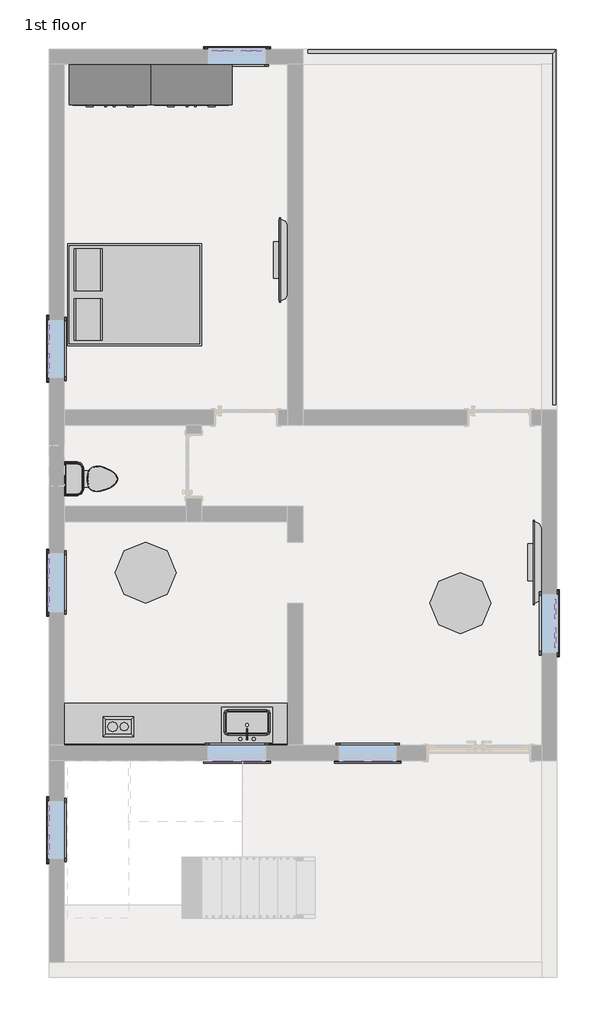
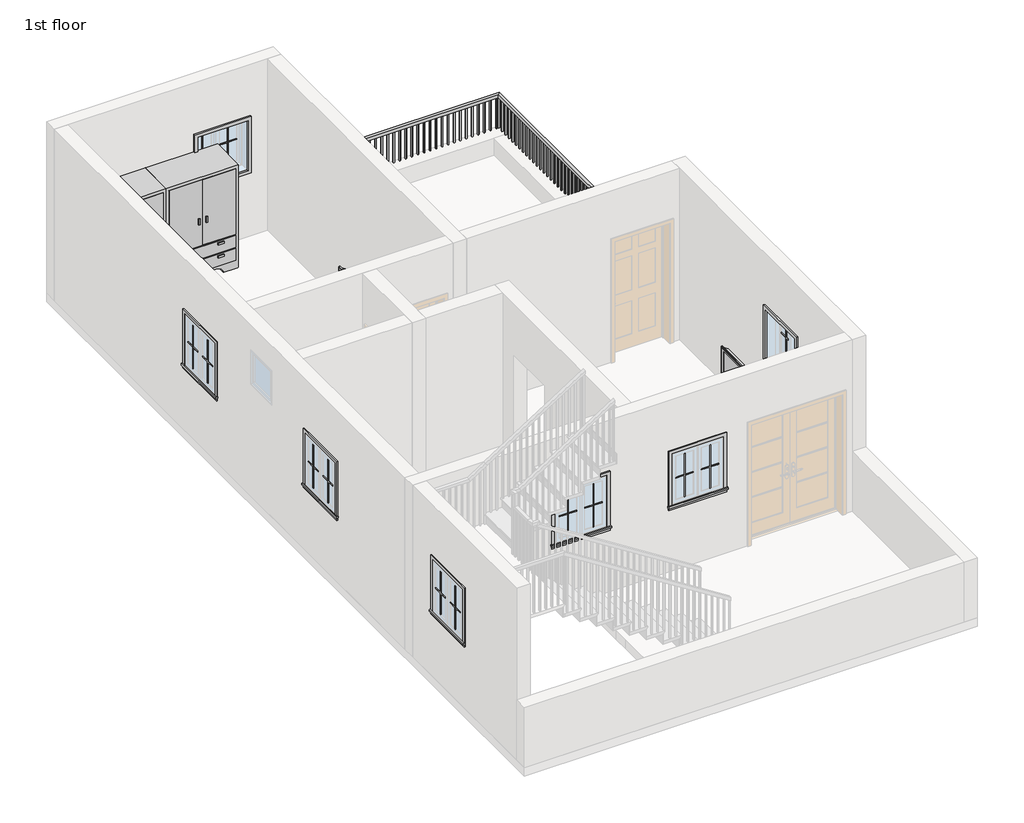
# One storey, part 3 of 3: 29 proxies, 8 furniture elements, 2 flow terminals, 1 railing.
"""IFC4 building model written with IfcOpenShell, lengths in millimetres."""

from ifc_helpers import new_model, si_unit, frame, origin, place, context, project, spatial, polyline, outline, extrude, faceted_brep, transform, mapped, element, save
from components import proxy_fb8a77b2, muntin_pattern_2x2_muntin_pattern_2x2_b3fe6957, muntin_pattern_2x2_muntin_pattern_2x2_3e0ecaf2, trim_window_exterior_flat_with_sill_41619996, trim_window_interior_flat_picture_frame_51c85655, flow_terminal_4d548711, toilet_domestic_3d_toilet_domestic_3d_ba6479b0, toilet_domestic_3d_toilet_domestic_3d_30431060, furniture_0315470b, furniture_691b2c5f, furniture_0b81fedb, furniture_ec754799, furniture_52f35bf4, furniture_82e269c4

model = new_model("IFC4")

# Units and contexts
model_context = context("Model", 3, world=origin())
ifc_project = project(units=[si_unit("LENGTHUNIT", "METRE", prefix="MILLI")], contexts=[model_context])

# Site, building, storey
site = spatial("IfcSite", under=ifc_project)
building = spatial("IfcBuilding", under=site)
storey = spatial("IfcBuildingStorey", under=building, Name="1st floor", Elevation=3810.0)

# Proxies
placement = place(None, origin())
proxy_shape = proxy_fb8a77b2(model_context)
element("IfcBuildingElementProxy", 1, Name="Cook Top-2 Unit : 12\" x 18\"", ObjectType="Cook Top-2 Unit : 12\" x 18\"", at=placement, inside=storey, context=model_context, shape_type="MappedRepresentation", body=[
    mapped(proxy_shape, transform((20084.9384757, 6960.5752787, 3810.0), x_axis=(0.0, 1.0, 0.0), y_axis=(-1.0, 0.0, 0.0), z_axis=(0.0, 0.0, 1.0))),
])
muntin_pattern_2x2_muntin_pattern_2x2_shape = muntin_pattern_2x2_muntin_pattern_2x2_b3fe6957(model_context)
element("IfcBuildingElementProxy", 2, Name="Muntin Pattern_2x2 : Muntin Pattern_2x2", ObjectType="Muntin Pattern_2x2 : Muntin Pattern_2x2", at=placement, inside=storey, context=model_context, shape_type="MappedRepresentation", body=[
    mapped(muntin_pattern_2x2_muntin_pattern_2x2_shape, transform((19022.8386801, 8981.4627787, 5064.125), x_axis=(0.0, 1.0, 0.0), y_axis=(-1.0, 0.0, 0.0), z_axis=(0.0, 0.0, 1.0))),
])
element("IfcBuildingElementProxy", 3, Name="Muntin Pattern_2x2 : Muntin Pattern_2x2", ObjectType="Muntin Pattern_2x2 : Muntin Pattern_2x2", at=placement, inside=storey, context=model_context, shape_type="MappedRepresentation", body=[
    mapped(muntin_pattern_2x2_muntin_pattern_2x2_shape, transform((19022.8386801, 12486.6627787, 5064.125), x_axis=(0.0, 1.0, 0.0), y_axis=(-1.0, 0.0, 0.0), z_axis=(0.0, 0.0, 1.0))),
])
element("IfcBuildingElementProxy", 4, Name="Muntin Pattern_2x2 : Muntin Pattern_2x2", ObjectType="Muntin Pattern_2x2 : Muntin Pattern_2x2", at=placement, inside=storey, context=model_context, shape_type="MappedRepresentation", body=[
    mapped(muntin_pattern_2x2_muntin_pattern_2x2_shape, transform((26623.7886801, 8800.4877787, 5064.125), x_axis=(0.0, -1.0, 0.0), y_axis=(1.0, 0.0, 0.0), z_axis=(0.0, 0.0, 1.0))),
])
element("IfcBuildingElementProxy", 5, Name="Muntin Pattern_2x2 : Muntin Pattern_2x2", ObjectType="Muntin Pattern_2x2 : Muntin Pattern_2x2", at=placement, inside=storey, context=model_context, shape_type="MappedRepresentation", body=[
    mapped(muntin_pattern_2x2_muntin_pattern_2x2_shape, transform((21618.4011801, 17187.2502787, 5064.125), x_axis=(1.0, 0.0, 0.0), y_axis=(0.0, 1.0, 0.0), z_axis=(0.0, 0.0, 1.0))),
])
element("IfcBuildingElementProxy", 6, Name="Muntin Pattern_2x2 : Muntin Pattern_2x2", ObjectType="Muntin Pattern_2x2 : Muntin Pattern_2x2", at=placement, inside=storey, context=model_context, shape_type="MappedRepresentation", body=[
    mapped(muntin_pattern_2x2_muntin_pattern_2x2_shape, transform((22047.0261801, 6538.3002787, 5064.125), x_axis=(-1.0, 0.0, 0.0), y_axis=(0.0, -1.0, 0.0), z_axis=(0.0, 0.0, 1.0))),
])
element("IfcBuildingElementProxy", 7, Name="Muntin Pattern_2x2 : Muntin Pattern_2x2", ObjectType="Muntin Pattern_2x2 : Muntin Pattern_2x2", at=placement, inside=storey, context=model_context, shape_type="MappedRepresentation", body=[
    mapped(muntin_pattern_2x2_muntin_pattern_2x2_shape, transform((24009.1761801, 6538.3002787, 5064.125), x_axis=(-1.0, 0.0, 0.0), y_axis=(0.0, -1.0, 0.0), z_axis=(0.0, 0.0, 1.0))),
])
element("IfcBuildingElementProxy", 8, Name="Muntin Pattern_2x2 : Muntin Pattern_2x2", ObjectType="Muntin Pattern_2x2 : Muntin Pattern_2x2", at=placement, inside=storey, context=model_context, shape_type="MappedRepresentation", body=[
    mapped(muntin_pattern_2x2_muntin_pattern_2x2_shape, transform((19022.8386801, 5273.0627787, 5064.125), x_axis=(0.0, 1.0, 0.0), y_axis=(-1.0, 0.0, 0.0), z_axis=(0.0, 0.0, 1.0))),
])
muntin_pattern_2x2_muntin_pattern_2x2_2_shape = muntin_pattern_2x2_muntin_pattern_2x2_3e0ecaf2(model_context)
element("IfcBuildingElementProxy", 9, Name="Muntin Pattern_2x2 : Muntin Pattern_2x2", ObjectType="Muntin Pattern_2x2 : Muntin Pattern_2x2", at=placement, inside=storey, context=model_context, shape_type="MappedRepresentation", body=[
    mapped(muntin_pattern_2x2_muntin_pattern_2x2_2_shape, transform((19022.8386801, 9410.0877787, 5064.125), x_axis=(0.0, -1.0, 0.0), y_axis=(1.0, 0.0, 0.0), z_axis=(0.0, 0.0, 1.0))),
])
element("IfcBuildingElementProxy", 10, Name="Muntin Pattern_2x2 : Muntin Pattern_2x2", ObjectType="Muntin Pattern_2x2 : Muntin Pattern_2x2", at=placement, inside=storey, context=model_context, shape_type="MappedRepresentation", body=[
    mapped(muntin_pattern_2x2_muntin_pattern_2x2_2_shape, transform((19022.8386801, 12915.2877787, 5064.125), x_axis=(0.0, -1.0, 0.0), y_axis=(1.0, 0.0, 0.0), z_axis=(0.0, 0.0, 1.0))),
])
element("IfcBuildingElementProxy", 11, Name="Muntin Pattern_2x2 : Muntin Pattern_2x2", ObjectType="Muntin Pattern_2x2 : Muntin Pattern_2x2", at=placement, inside=storey, context=model_context, shape_type="MappedRepresentation", body=[
    mapped(muntin_pattern_2x2_muntin_pattern_2x2_2_shape, transform((26623.7886801, 8371.8627787, 5064.125), x_axis=(0.0, 1.0, 0.0), y_axis=(-1.0, 0.0, 0.0), z_axis=(0.0, 0.0, 1.0))),
])
element("IfcBuildingElementProxy", 12, Name="Muntin Pattern_2x2 : Muntin Pattern_2x2", ObjectType="Muntin Pattern_2x2 : Muntin Pattern_2x2", at=placement, inside=storey, context=model_context, shape_type="MappedRepresentation", body=[
    mapped(muntin_pattern_2x2_muntin_pattern_2x2_2_shape, transform((22047.0261801, 17187.2502787, 5064.125), x_axis=(-1.0, 0.0, 0.0), y_axis=(0.0, -1.0, 0.0), z_axis=(0.0, 0.0, 1.0))),
])
element("IfcBuildingElementProxy", 13, Name="Muntin Pattern_2x2 : Muntin Pattern_2x2", ObjectType="Muntin Pattern_2x2 : Muntin Pattern_2x2", at=placement, inside=storey, context=model_context, shape_type="MappedRepresentation", body=[
    mapped(muntin_pattern_2x2_muntin_pattern_2x2_2_shape, transform((21618.4011801, 6538.3002787, 5064.125), x_axis=(1.0, 0.0, 0.0), y_axis=(0.0, 1.0, 0.0), z_axis=(0.0, 0.0, 1.0))),
])
element("IfcBuildingElementProxy", 14, Name="Muntin Pattern_2x2 : Muntin Pattern_2x2", ObjectType="Muntin Pattern_2x2 : Muntin Pattern_2x2", at=placement, inside=storey, context=model_context, shape_type="MappedRepresentation", body=[
    mapped(muntin_pattern_2x2_muntin_pattern_2x2_2_shape, transform((23580.5511801, 6538.3002787, 5064.125), x_axis=(1.0, 0.0, 0.0), y_axis=(0.0, 1.0, 0.0), z_axis=(0.0, 0.0, 1.0))),
])
element("IfcBuildingElementProxy", 15, Name="Muntin Pattern_2x2 : Muntin Pattern_2x2", ObjectType="Muntin Pattern_2x2 : Muntin Pattern_2x2", at=placement, inside=storey, context=model_context, shape_type="MappedRepresentation", body=[
    mapped(muntin_pattern_2x2_muntin_pattern_2x2_2_shape, transform((19022.8386801, 5701.6877787, 5064.125), x_axis=(0.0, -1.0, 0.0), y_axis=(1.0, 0.0, 0.0), z_axis=(0.0, 0.0, 1.0))),
])
trim_window_exterior_flat_with_sill_shape = trim_window_exterior_flat_with_sill_41619996(model_context)
element("IfcBuildingElementProxy", 16, Name="Trim-Window-Exterior-Flat : with Sill", ObjectType="Trim-Window-Exterior-Flat : with Sill", at=placement, inside=storey, context=model_context, shape_type="MappedRepresentation", body=[
    mapped(trim_window_exterior_flat_with_sill_shape, transform((19013.3136801, 9195.7752787, 5908.675), x_axis=(0.0, -1.0, 0.0), y_axis=(0.0, 0.0, 1.0), z_axis=(-1.0, 0.0, 0.0))),
])
element("IfcBuildingElementProxy", 17, Name="Trim-Window-Exterior-Flat : with Sill", ObjectType="Trim-Window-Exterior-Flat : with Sill", at=placement, inside=storey, context=model_context, shape_type="MappedRepresentation", body=[
    mapped(trim_window_exterior_flat_with_sill_shape, transform((19013.3136801, 12700.9752787, 5908.675), x_axis=(0.0, -1.0, 0.0), y_axis=(0.0, 0.0, 1.0), z_axis=(-1.0, 0.0, 0.0))),
])
element("IfcBuildingElementProxy", 18, Name="Trim-Window-Exterior-Flat : with Sill", ObjectType="Trim-Window-Exterior-Flat : with Sill", at=placement, inside=storey, context=model_context, shape_type="MappedRepresentation", body=[
    mapped(trim_window_exterior_flat_with_sill_shape, transform((26633.3136801, 8586.1752787, 5908.675), x_axis=(0.0, 1.0, 0.0), y_axis=(0.0, 0.0, 1.0), z_axis=(1.0, 0.0, 0.0))),
])
element("IfcBuildingElementProxy", 19, Name="Trim-Window-Exterior-Flat : with Sill", ObjectType="Trim-Window-Exterior-Flat : with Sill", at=placement, inside=storey, context=model_context, shape_type="MappedRepresentation", body=[
    mapped(trim_window_exterior_flat_with_sill_shape, transform((21832.7136801, 17196.7752787, 5908.675), x_axis=(-1.0, 0.0, 0.0), y_axis=(0.0, 0.0, 1.0), z_axis=(0.0, 1.0, 0.0))),
])
element("IfcBuildingElementProxy", 20, Name="Trim-Window-Exterior-Flat : with Sill", ObjectType="Trim-Window-Exterior-Flat : with Sill", at=placement, inside=storey, context=model_context, shape_type="MappedRepresentation", body=[
    mapped(trim_window_exterior_flat_with_sill_shape, transform((21832.7136801, 6528.7752787, 5908.675), x_axis=(1.0, 0.0, 0.0), y_axis=(0.0, 0.0, 1.0), z_axis=(0.0, -1.0, 0.0))),
])
element("IfcBuildingElementProxy", 21, Name="Trim-Window-Exterior-Flat : with Sill", ObjectType="Trim-Window-Exterior-Flat : with Sill", at=placement, inside=storey, context=model_context, shape_type="MappedRepresentation", body=[
    mapped(trim_window_exterior_flat_with_sill_shape, transform((23794.8636801, 6528.7752787, 5908.675), x_axis=(1.0, 0.0, 0.0), y_axis=(0.0, 0.0, 1.0), z_axis=(0.0, -1.0, 0.0))),
])
element("IfcBuildingElementProxy", 22, Name="Trim-Window-Exterior-Flat : with Sill", ObjectType="Trim-Window-Exterior-Flat : with Sill", at=placement, inside=storey, context=model_context, shape_type="MappedRepresentation", body=[
    mapped(trim_window_exterior_flat_with_sill_shape, transform((19013.3136801, 5487.3752787, 5908.675), x_axis=(0.0, -1.0, 0.0), y_axis=(0.0, 0.0, 1.0), z_axis=(-1.0, 0.0, 0.0))),
])
trim_window_interior_flat_picture_frame_shape = trim_window_interior_flat_picture_frame_51c85655(model_context)
element("IfcBuildingElementProxy", 23, Name="Trim-Window-Interior-Flat : Picture Frame", ObjectType="Trim-Window-Interior-Flat : Picture Frame", at=placement, inside=storey, context=model_context, shape_type="MappedRepresentation", body=[
    mapped(trim_window_interior_flat_picture_frame_shape, transform((19241.9136801, 9195.7752787, 5908.675), x_axis=(0.0, 1.0, 0.0), y_axis=(0.0, 0.0, 1.0), z_axis=(1.0, 0.0, 0.0))),
])
element("IfcBuildingElementProxy", 24, Name="Trim-Window-Interior-Flat : Picture Frame", ObjectType="Trim-Window-Interior-Flat : Picture Frame", at=placement, inside=storey, context=model_context, shape_type="MappedRepresentation", body=[
    mapped(trim_window_interior_flat_picture_frame_shape, transform((19241.9136801, 12700.9752787, 5908.675), x_axis=(0.0, 1.0, 0.0), y_axis=(0.0, 0.0, 1.0), z_axis=(1.0, 0.0, 0.0))),
])
element("IfcBuildingElementProxy", 25, Name="Trim-Window-Interior-Flat : Picture Frame", ObjectType="Trim-Window-Interior-Flat : Picture Frame", at=placement, inside=storey, context=model_context, shape_type="MappedRepresentation", body=[
    mapped(trim_window_interior_flat_picture_frame_shape, transform((26404.7136801, 8586.1752787, 5908.675), x_axis=(0.0, -1.0, 0.0), y_axis=(0.0, 0.0, 1.0), z_axis=(-1.0, 0.0, 0.0))),
])
element("IfcBuildingElementProxy", 26, Name="Trim-Window-Interior-Flat : Picture Frame", ObjectType="Trim-Window-Interior-Flat : Picture Frame", at=placement, inside=storey, context=model_context, shape_type="MappedRepresentation", body=[
    mapped(trim_window_interior_flat_picture_frame_shape, transform((21832.7136801, 16968.1752787, 5908.675), x_axis=(1.0, 0.0, 0.0), y_axis=(0.0, 0.0, 1.0), z_axis=(0.0, -1.0, 0.0))),
])
element("IfcBuildingElementProxy", 27, Name="Trim-Window-Interior-Flat : Picture Frame", ObjectType="Trim-Window-Interior-Flat : Picture Frame", at=placement, inside=storey, context=model_context, shape_type="MappedRepresentation", body=[
    mapped(trim_window_interior_flat_picture_frame_shape, transform((21832.7136801, 6757.3752787, 5908.675), x_axis=(-1.0, 0.0, 0.0), y_axis=(0.0, 0.0, 1.0), z_axis=(0.0, 1.0, 0.0))),
])
element("IfcBuildingElementProxy", 28, Name="Trim-Window-Interior-Flat : Picture Frame", ObjectType="Trim-Window-Interior-Flat : Picture Frame", at=placement, inside=storey, context=model_context, shape_type="MappedRepresentation", body=[
    mapped(trim_window_interior_flat_picture_frame_shape, transform((23794.8636801, 6757.3752787, 5908.675), x_axis=(-1.0, 0.0, 0.0), y_axis=(0.0, 0.0, 1.0), z_axis=(0.0, 1.0, 0.0))),
])
element("IfcBuildingElementProxy", 29, Name="Trim-Window-Interior-Flat : Picture Frame", ObjectType="Trim-Window-Interior-Flat : Picture Frame", at=placement, inside=storey, context=model_context, shape_type="MappedRepresentation", body=[
    mapped(trim_window_interior_flat_picture_frame_shape, transform((19241.9136801, 5487.3752787, 5908.675), x_axis=(0.0, 1.0, 0.0), y_axis=(0.0, 0.0, 1.0), z_axis=(1.0, 0.0, 0.0))),
])

# Flow terminals
flow_terminal_shape = flow_terminal_4d548711(model_context)
element("IfcFlowTerminal", 30, ObjectType="Sink Kitchen-Single : 30\" x 21\"", at=placement, inside=storey, context=model_context, shape_type="MappedRepresentation", body=[
    mapped(flow_terminal_shape, transform((22000.8029206, 7064.5206798, 3810.0), x_axis=(-1.0, 0.0, 0.0), y_axis=(0.0, -1.0, 0.0), z_axis=(0.0, 0.0, 1.0))),
])
toilet_domestic_3d_toilet_domestic_3d_shape = toilet_domestic_3d_toilet_domestic_3d_ba6479b0(model_context)
toilet_domestic_3d_toilet_domestic_3d_2_shape = toilet_domestic_3d_toilet_domestic_3d_30431060(model_context)
element("IfcFlowTerminal", 31, ObjectType="Toilet-Domestic-3D : Toilet-Domestic-3D", at=placement, inside=storey, context=model_context, shape_type="MappedRepresentation", body=[
    mapped(toilet_domestic_3d_toilet_domestic_3d_shape, transform((19736.6097074, 10752.6409313, 3810.0), x_axis=(0.0, 1.0, 0.0), y_axis=(-1.0, 0.0, 0.0), z_axis=(0.0, 0.0, 1.0))),
    mapped(toilet_domestic_3d_toilet_domestic_3d_2_shape, transform((19736.6097074, 10752.6409313, 3810.0), x_axis=(0.0, 1.0, 0.0), y_axis=(-1.0, 0.0, 0.0), z_axis=(0.0, 0.0, 1.0))),
])

# Furniture
furniture_shape = furniture_0315470b(model_context)
element("IfcFurniture", 32, ObjectType="Bed-Box : Queen 60\" x 79\"", at=placement, inside=storey, context=model_context, shape_type="MappedRepresentation", body=[
    mapped(furniture_shape, transform((20061.5841719, 13174.6228197, 3810.0), x_axis=(0.0, 1.0, 0.0), y_axis=(-1.0, 0.0, 0.0), z_axis=(0.0, 0.0, 1.0))),
])
furniture_2_shape = furniture_691b2c5f(model_context)
element("IfcFurniture", 33, ObjectType="Counter Top w Sink Hole : 24\" Depth", at=placement, inside=storey, context=model_context, shape_type="MappedRepresentation", body=[
    mapped(furniture_2_shape, transform((21394.251385, 6757.3752787, 3810.0), x_axis=(-1.0, 0.0, 0.0), y_axis=(0.0, -1.0, 0.0), z_axis=(0.0, 0.0, 1.0))),
])
furniture_3_shape = furniture_0b81fedb(model_context)
element("IfcFurniture", 34, ObjectType="TV - Flat Screen : 50\"", at=placement, inside=storey, context=model_context, shape_type="MappedRepresentation", body=[
    mapped(furniture_3_shape, transform((26346.1750564, 9496.6307646, 3810.0), x_axis=(0.0, -1.0, 0.0), y_axis=(1.0, 0.0, 0.0), z_axis=(0.0, 0.0, 1.0))),
])
element("IfcFurniture", 35, ObjectType="TV - Flat Screen : 50\"", at=placement, inside=storey, context=model_context, shape_type="MappedRepresentation", body=[
    mapped(furniture_3_shape, transform((22536.1750564, 14030.5307646, 3810.0), x_axis=(0.0, -1.0, 0.0), y_axis=(1.0, 0.0, 0.0), z_axis=(0.0, 0.0, 1.0))),
])
furniture_4_shape = furniture_ec754799(model_context)
element("IfcFurniture", 36, ObjectType="Table-Dining Round : 36\" Diameter", at=placement, inside=storey, context=model_context, shape_type="MappedRepresentation", body=[
    mapped(furniture_4_shape, transform((25081.8317129, 9075.8539672, 3810.0), x_axis=(1.0, 0.0, 0.0), y_axis=(0.0, 1.0, 0.0), z_axis=(0.0, 0.0, 1.0))),
])
furniture_5_shape = furniture_52f35bf4(model_context)
element("IfcFurniture", 37, ObjectType="Table-Dining Round w Chairs : 36\" Diameter", at=placement, inside=storey, context=model_context, shape_type="MappedRepresentation", body=[
    mapped(furniture_5_shape, transform((20357.4317129, 9533.0539672, 3810.0), x_axis=(1.0, 0.0, 0.0), y_axis=(0.0, 1.0, 0.0), z_axis=(0.0, 0.0, 1.0))),
])
furniture_6_shape = furniture_82e269c4(model_context)
element("IfcFurniture", 38, ObjectType="Wardrobe : 48\" x 72\" x 24\"", at=placement, inside=storey, context=model_context, shape_type="MappedRepresentation", body=[
    mapped(furniture_6_shape, transform((20196.9069399, 17247.1140883, 3810.0), x_axis=(1.0, 0.0, 0.0), y_axis=(0.0, 1.0, 0.0), z_axis=(0.0, 0.0, 1.0))),
])
element("IfcFurniture", 39, ObjectType="Wardrobe : 48\" x 72\" x 24\"", at=placement, inside=storey, context=model_context, shape_type="MappedRepresentation", body=[
    mapped(furniture_6_shape, transform((21416.1069399, 17247.1140883, 3810.0), x_axis=(1.0, 0.0, 0.0), y_axis=(0.0, 1.0, 0.0), z_axis=(0.0, 0.0, 1.0))),
])

# Railing
element("IfcRailing", 40, ObjectType="Handrail - Rectangular", at=placement, inside=storey, context=model_context, shape_type="SolidModel", body=[
    faceted_brep([(22899.5136801, 17184.0752787, 4724.4), (22899.5136801, 17184.0752787, 4673.6), (22899.5136801, 17133.2752787, 4673.6), (22899.5136801, 17133.2752787, 4724.4), (26620.6136801, 17184.0752787, 4724.4), (26620.6136801, 17184.0752787, 4673.6), (26569.8136801, 17133.2752787, 4673.6), (26569.8136801, 17133.2752787, 4724.4), (26620.6136801, 11862.7752787, 4724.4), (26569.8136801, 11862.7752787, 4724.4), (26569.8136801, 11862.7752787, 4673.6), (26620.6136801, 11862.7752787, 4673.6)], [[[0, 1, 2, 3]], [[1, 0, 4, 5]], [[2, 1, 5, 6]], [[3, 2, 6, 7]], [[0, 3, 7, 4]], [[8, 9, 10, 11]], [[5, 4, 8, 11]], [[6, 5, 11, 10]], [[7, 6, 10, 9]], [[4, 7, 9, 8]]]),
    extrude(outline(polyline([(26604.7386801, 11885.0002787), (26604.7386801, 11865.9502787), (26585.6886801, 11865.9502787), (26585.6886801, 11885.0002787), (26604.7386801, 11885.0002787)])), frame((0.0, 0.0, 3810.0), z_axis=(0.0, 0.0, 1.0), x_axis=(1.0, 0.0, 0.0)), (0.0, 0.0, 1.0), 863.6),
    extrude(outline(polyline([(26604.7386801, 11986.6002787), (26604.7386801, 11967.5502787), (26585.6886801, 11967.5502787), (26585.6886801, 11986.6002787), (26604.7386801, 11986.6002787)])), frame((0.0, 0.0, 3810.0), z_axis=(0.0, 0.0, 1.0), x_axis=(1.0, 0.0, 0.0)), (0.0, 0.0, 1.0), 863.6),
    extrude(outline(polyline([(26604.7386801, 12088.2002787), (26604.7386801, 12069.1502787), (26585.6886801, 12069.1502787), (26585.6886801, 12088.2002787), (26604.7386801, 12088.2002787)])), frame((0.0, 0.0, 3810.0), z_axis=(0.0, 0.0, 1.0), x_axis=(1.0, 0.0, 0.0)), (0.0, 0.0, 1.0), 863.6),
    extrude(outline(polyline([(26604.7386801, 12189.8002787), (26604.7386801, 12170.7502787), (26585.6886801, 12170.7502787), (26585.6886801, 12189.8002787), (26604.7386801, 12189.8002787)])), frame((0.0, 0.0, 3810.0), z_axis=(0.0, 0.0, 1.0), x_axis=(1.0, 0.0, 0.0)), (0.0, 0.0, 1.0), 863.6),
    extrude(outline(polyline([(26604.7386801, 12291.4002787), (26604.7386801, 12272.3502787), (26585.6886801, 12272.3502787), (26585.6886801, 12291.4002787), (26604.7386801, 12291.4002787)])), frame((0.0, 0.0, 3810.0), z_axis=(0.0, 0.0, 1.0), x_axis=(1.0, 0.0, 0.0)), (0.0, 0.0, 1.0), 863.6),
    extrude(outline(polyline([(26604.7386801, 12393.0002787), (26604.7386801, 12373.9502787), (26585.6886801, 12373.9502787), (26585.6886801, 12393.0002787), (26604.7386801, 12393.0002787)])), frame((0.0, 0.0, 3810.0), z_axis=(0.0, 0.0, 1.0), x_axis=(1.0, 0.0, 0.0)), (0.0, 0.0, 1.0), 863.6),
    extrude(outline(polyline([(26604.7386801, 12494.6002787), (26604.7386801, 12475.5502787), (26585.6886801, 12475.5502787), (26585.6886801, 12494.6002787), (26604.7386801, 12494.6002787)])), frame((0.0, 0.0, 3810.0), z_axis=(0.0, 0.0, 1.0), x_axis=(1.0, 0.0, 0.0)), (0.0, 0.0, 1.0), 863.6),
    extrude(outline(polyline([(26604.7386801, 12596.2002787), (26604.7386801, 12577.1502787), (26585.6886801, 12577.1502787), (26585.6886801, 12596.2002787), (26604.7386801, 12596.2002787)])), frame((0.0, 0.0, 3810.0), z_axis=(0.0, 0.0, 1.0), x_axis=(1.0, 0.0, 0.0)), (0.0, 0.0, 1.0), 863.6),
    extrude(outline(polyline([(26604.7386801, 12697.8002787), (26604.7386801, 12678.7502787), (26585.6886801, 12678.7502787), (26585.6886801, 12697.8002787), (26604.7386801, 12697.8002787)])), frame((0.0, 0.0, 3810.0), z_axis=(0.0, 0.0, 1.0), x_axis=(1.0, 0.0, 0.0)), (0.0, 0.0, 1.0), 863.6),
    extrude(outline(polyline([(26604.7386801, 12799.4002787), (26604.7386801, 12780.3502787), (26585.6886801, 12780.3502787), (26585.6886801, 12799.4002787), (26604.7386801, 12799.4002787)])), frame((0.0, 0.0, 3810.0), z_axis=(0.0, 0.0, 1.0), x_axis=(1.0, 0.0, 0.0)), (0.0, 0.0, 1.0), 863.6),
    extrude(outline(polyline([(26604.7386801, 12901.0002787), (26604.7386801, 12881.9502787), (26585.6886801, 12881.9502787), (26585.6886801, 12901.0002787), (26604.7386801, 12901.0002787)])), frame((0.0, 0.0, 3810.0), z_axis=(0.0, 0.0, 1.0), x_axis=(1.0, 0.0, 0.0)), (0.0, 0.0, 1.0), 863.6),
    extrude(outline(polyline([(26604.7386801, 13002.6002787), (26604.7386801, 12983.5502787), (26585.6886801, 12983.5502787), (26585.6886801, 13002.6002787), (26604.7386801, 13002.6002787)])), frame((0.0, 0.0, 3810.0), z_axis=(0.0, 0.0, 1.0), x_axis=(1.0, 0.0, 0.0)), (0.0, 0.0, 1.0), 863.6),
    extrude(outline(polyline([(26604.7386801, 13104.2002787), (26604.7386801, 13085.1502787), (26585.6886801, 13085.1502787), (26585.6886801, 13104.2002787), (26604.7386801, 13104.2002787)])), frame((0.0, 0.0, 3810.0), z_axis=(0.0, 0.0, 1.0), x_axis=(1.0, 0.0, 0.0)), (0.0, 0.0, 1.0), 863.6),
    extrude(outline(polyline([(26604.7386801, 13205.8002787), (26604.7386801, 13186.7502787), (26585.6886801, 13186.7502787), (26585.6886801, 13205.8002787), (26604.7386801, 13205.8002787)])), frame((0.0, 0.0, 3810.0), z_axis=(0.0, 0.0, 1.0), x_axis=(1.0, 0.0, 0.0)), (0.0, 0.0, 1.0), 863.6),
    extrude(outline(polyline([(26604.7386801, 13307.4002787), (26604.7386801, 13288.3502787), (26585.6886801, 13288.3502787), (26585.6886801, 13307.4002787), (26604.7386801, 13307.4002787)])), frame((0.0, 0.0, 3810.0), z_axis=(0.0, 0.0, 1.0), x_axis=(1.0, 0.0, 0.0)), (0.0, 0.0, 1.0), 863.6),
    extrude(outline(polyline([(26604.7386801, 13409.0002787), (26604.7386801, 13389.9502787), (26585.6886801, 13389.9502787), (26585.6886801, 13409.0002787), (26604.7386801, 13409.0002787)])), frame((0.0, 0.0, 3810.0), z_axis=(0.0, 0.0, 1.0), x_axis=(1.0, 0.0, 0.0)), (0.0, 0.0, 1.0), 863.6),
    extrude(outline(polyline([(26604.7386801, 13510.6002787), (26604.7386801, 13491.5502787), (26585.6886801, 13491.5502787), (26585.6886801, 13510.6002787), (26604.7386801, 13510.6002787)])), frame((0.0, 0.0, 3810.0), z_axis=(0.0, 0.0, 1.0), x_axis=(1.0, 0.0, 0.0)), (0.0, 0.0, 1.0), 863.6),
    extrude(outline(polyline([(26604.7386801, 13612.2002787), (26604.7386801, 13593.1502787), (26585.6886801, 13593.1502787), (26585.6886801, 13612.2002787), (26604.7386801, 13612.2002787)])), frame((0.0, 0.0, 3810.0), z_axis=(0.0, 0.0, 1.0), x_axis=(1.0, 0.0, 0.0)), (0.0, 0.0, 1.0), 863.6),
    extrude(outline(polyline([(26604.7386801, 13713.8002787), (26604.7386801, 13694.7502787), (26585.6886801, 13694.7502787), (26585.6886801, 13713.8002787), (26604.7386801, 13713.8002787)])), frame((0.0, 0.0, 3810.0), z_axis=(0.0, 0.0, 1.0), x_axis=(1.0, 0.0, 0.0)), (0.0, 0.0, 1.0), 863.6),
    extrude(outline(polyline([(26604.7386801, 13815.4002787), (26604.7386801, 13796.3502787), (26585.6886801, 13796.3502787), (26585.6886801, 13815.4002787), (26604.7386801, 13815.4002787)])), frame((0.0, 0.0, 3810.0), z_axis=(0.0, 0.0, 1.0), x_axis=(1.0, 0.0, 0.0)), (0.0, 0.0, 1.0), 863.6),
    extrude(outline(polyline([(26604.7386801, 13917.0002787), (26604.7386801, 13897.9502787), (26585.6886801, 13897.9502787), (26585.6886801, 13917.0002787), (26604.7386801, 13917.0002787)])), frame((0.0, 0.0, 3810.0), z_axis=(0.0, 0.0, 1.0), x_axis=(1.0, 0.0, 0.0)), (0.0, 0.0, 1.0), 863.6),
    extrude(outline(polyline([(26604.7386801, 14018.6002787), (26604.7386801, 13999.5502787), (26585.6886801, 13999.5502787), (26585.6886801, 14018.6002787), (26604.7386801, 14018.6002787)])), frame((0.0, 0.0, 3810.0), z_axis=(0.0, 0.0, 1.0), x_axis=(1.0, 0.0, 0.0)), (0.0, 0.0, 1.0), 863.6),
    extrude(outline(polyline([(26604.7386801, 14120.2002787), (26604.7386801, 14101.1502787), (26585.6886801, 14101.1502787), (26585.6886801, 14120.2002787), (26604.7386801, 14120.2002787)])), frame((0.0, 0.0, 3810.0), z_axis=(0.0, 0.0, 1.0), x_axis=(1.0, 0.0, 0.0)), (0.0, 0.0, 1.0), 863.6),
    extrude(outline(polyline([(26604.7386801, 14221.8002787), (26604.7386801, 14202.7502787), (26585.6886801, 14202.7502787), (26585.6886801, 14221.8002787), (26604.7386801, 14221.8002787)])), frame((0.0, 0.0, 3810.0), z_axis=(0.0, 0.0, 1.0), x_axis=(1.0, 0.0, 0.0)), (0.0, 0.0, 1.0), 863.6),
    extrude(outline(polyline([(26604.7386801, 14323.4002787), (26604.7386801, 14304.3502787), (26585.6886801, 14304.3502787), (26585.6886801, 14323.4002787), (26604.7386801, 14323.4002787)])), frame((0.0, 0.0, 3810.0), z_axis=(0.0, 0.0, 1.0), x_axis=(1.0, 0.0, 0.0)), (0.0, 0.0, 1.0), 863.6),
    extrude(outline(polyline([(26604.7386801, 14425.0002787), (26604.7386801, 14405.9502787), (26585.6886801, 14405.9502787), (26585.6886801, 14425.0002787), (26604.7386801, 14425.0002787)])), frame((0.0, 0.0, 3810.0), z_axis=(0.0, 0.0, 1.0), x_axis=(1.0, 0.0, 0.0)), (0.0, 0.0, 1.0), 863.6),
    extrude(outline(polyline([(26604.7386801, 14526.6002787), (26604.7386801, 14507.5502787), (26585.6886801, 14507.5502787), (26585.6886801, 14526.6002787), (26604.7386801, 14526.6002787)])), frame((0.0, 0.0, 3810.0), z_axis=(0.0, 0.0, 1.0), x_axis=(1.0, 0.0, 0.0)), (0.0, 0.0, 1.0), 863.6),
    extrude(outline(polyline([(26604.7386801, 14628.2002787), (26604.7386801, 14609.1502787), (26585.6886801, 14609.1502787), (26585.6886801, 14628.2002787), (26604.7386801, 14628.2002787)])), frame((0.0, 0.0, 3810.0), z_axis=(0.0, 0.0, 1.0), x_axis=(1.0, 0.0, 0.0)), (0.0, 0.0, 1.0), 863.6),
    extrude(outline(polyline([(26604.7386801, 14729.8002787), (26604.7386801, 14710.7502787), (26585.6886801, 14710.7502787), (26585.6886801, 14729.8002787), (26604.7386801, 14729.8002787)])), frame((0.0, 0.0, 3810.0), z_axis=(0.0, 0.0, 1.0), x_axis=(1.0, 0.0, 0.0)), (0.0, 0.0, 1.0), 863.6),
    extrude(outline(polyline([(26604.7386801, 14831.4002787), (26604.7386801, 14812.3502787), (26585.6886801, 14812.3502787), (26585.6886801, 14831.4002787), (26604.7386801, 14831.4002787)])), frame((0.0, 0.0, 3810.0), z_axis=(0.0, 0.0, 1.0), x_axis=(1.0, 0.0, 0.0)), (0.0, 0.0, 1.0), 863.6),
    extrude(outline(polyline([(26604.7386801, 14933.0002787), (26604.7386801, 14913.9502787), (26585.6886801, 14913.9502787), (26585.6886801, 14933.0002787), (26604.7386801, 14933.0002787)])), frame((0.0, 0.0, 3810.0), z_axis=(0.0, 0.0, 1.0), x_axis=(1.0, 0.0, 0.0)), (0.0, 0.0, 1.0), 863.6),
    extrude(outline(polyline([(26604.7386801, 15034.6002787), (26604.7386801, 15015.5502787), (26585.6886801, 15015.5502787), (26585.6886801, 15034.6002787), (26604.7386801, 15034.6002787)])), frame((0.0, 0.0, 3810.0), z_axis=(0.0, 0.0, 1.0), x_axis=(1.0, 0.0, 0.0)), (0.0, 0.0, 1.0), 863.6),
    extrude(outline(polyline([(26604.7386801, 15136.2002787), (26604.7386801, 15117.1502787), (26585.6886801, 15117.1502787), (26585.6886801, 15136.2002787), (26604.7386801, 15136.2002787)])), frame((0.0, 0.0, 3810.0), z_axis=(0.0, 0.0, 1.0), x_axis=(1.0, 0.0, 0.0)), (0.0, 0.0, 1.0), 863.6),
    extrude(outline(polyline([(26604.7386801, 15237.8002787), (26604.7386801, 15218.7502787), (26585.6886801, 15218.7502787), (26585.6886801, 15237.8002787), (26604.7386801, 15237.8002787)])), frame((0.0, 0.0, 3810.0), z_axis=(0.0, 0.0, 1.0), x_axis=(1.0, 0.0, 0.0)), (0.0, 0.0, 1.0), 863.6),
    extrude(outline(polyline([(26604.7386801, 15339.4002787), (26604.7386801, 15320.3502787), (26585.6886801, 15320.3502787), (26585.6886801, 15339.4002787), (26604.7386801, 15339.4002787)])), frame((0.0, 0.0, 3810.0), z_axis=(0.0, 0.0, 1.0), x_axis=(1.0, 0.0, 0.0)), (0.0, 0.0, 1.0), 863.6),
    extrude(outline(polyline([(26604.7386801, 15441.0002787), (26604.7386801, 15421.9502787), (26585.6886801, 15421.9502787), (26585.6886801, 15441.0002787), (26604.7386801, 15441.0002787)])), frame((0.0, 0.0, 3810.0), z_axis=(0.0, 0.0, 1.0), x_axis=(1.0, 0.0, 0.0)), (0.0, 0.0, 1.0), 863.6),
    extrude(outline(polyline([(26604.7386801, 15542.6002787), (26604.7386801, 15523.5502787), (26585.6886801, 15523.5502787), (26585.6886801, 15542.6002787), (26604.7386801, 15542.6002787)])), frame((0.0, 0.0, 3810.0), z_axis=(0.0, 0.0, 1.0), x_axis=(1.0, 0.0, 0.0)), (0.0, 0.0, 1.0), 863.6),
    extrude(outline(polyline([(26604.7386801, 15644.2002787), (26604.7386801, 15625.1502787), (26585.6886801, 15625.1502787), (26585.6886801, 15644.2002787), (26604.7386801, 15644.2002787)])), frame((0.0, 0.0, 3810.0), z_axis=(0.0, 0.0, 1.0), x_axis=(1.0, 0.0, 0.0)), (0.0, 0.0, 1.0), 863.6),
    extrude(outline(polyline([(26604.7386801, 15745.8002787), (26604.7386801, 15726.7502787), (26585.6886801, 15726.7502787), (26585.6886801, 15745.8002787), (26604.7386801, 15745.8002787)])), frame((0.0, 0.0, 3810.0), z_axis=(0.0, 0.0, 1.0), x_axis=(1.0, 0.0, 0.0)), (0.0, 0.0, 1.0), 863.6),
    extrude(outline(polyline([(26604.7386801, 15847.4002787), (26604.7386801, 15828.3502787), (26585.6886801, 15828.3502787), (26585.6886801, 15847.4002787), (26604.7386801, 15847.4002787)])), frame((0.0, 0.0, 3810.0), z_axis=(0.0, 0.0, 1.0), x_axis=(1.0, 0.0, 0.0)), (0.0, 0.0, 1.0), 863.6),
    extrude(outline(polyline([(26604.7386801, 15949.0002787), (26604.7386801, 15929.9502787), (26585.6886801, 15929.9502787), (26585.6886801, 15949.0002787), (26604.7386801, 15949.0002787)])), frame((0.0, 0.0, 3810.0), z_axis=(0.0, 0.0, 1.0), x_axis=(1.0, 0.0, 0.0)), (0.0, 0.0, 1.0), 863.6),
    extrude(outline(polyline([(26604.7386801, 16050.6002787), (26604.7386801, 16031.5502787), (26585.6886801, 16031.5502787), (26585.6886801, 16050.6002787), (26604.7386801, 16050.6002787)])), frame((0.0, 0.0, 3810.0), z_axis=(0.0, 0.0, 1.0), x_axis=(1.0, 0.0, 0.0)), (0.0, 0.0, 1.0), 863.6),
    extrude(outline(polyline([(26604.7386801, 16152.2002787), (26604.7386801, 16133.1502787), (26585.6886801, 16133.1502787), (26585.6886801, 16152.2002787), (26604.7386801, 16152.2002787)])), frame((0.0, 0.0, 3810.0), z_axis=(0.0, 0.0, 1.0), x_axis=(1.0, 0.0, 0.0)), (0.0, 0.0, 1.0), 863.6),
    extrude(outline(polyline([(26604.7386801, 16253.8002787), (26604.7386801, 16234.7502787), (26585.6886801, 16234.7502787), (26585.6886801, 16253.8002787), (26604.7386801, 16253.8002787)])), frame((0.0, 0.0, 3810.0), z_axis=(0.0, 0.0, 1.0), x_axis=(1.0, 0.0, 0.0)), (0.0, 0.0, 1.0), 863.6),
    extrude(outline(polyline([(26604.7386801, 16355.4002787), (26604.7386801, 16336.3502787), (26585.6886801, 16336.3502787), (26585.6886801, 16355.4002787), (26604.7386801, 16355.4002787)])), frame((0.0, 0.0, 3810.0), z_axis=(0.0, 0.0, 1.0), x_axis=(1.0, 0.0, 0.0)), (0.0, 0.0, 1.0), 863.6),
    extrude(outline(polyline([(26604.7386801, 16457.0002787), (26604.7386801, 16437.9502787), (26585.6886801, 16437.9502787), (26585.6886801, 16457.0002787), (26604.7386801, 16457.0002787)])), frame((0.0, 0.0, 3810.0), z_axis=(0.0, 0.0, 1.0), x_axis=(1.0, 0.0, 0.0)), (0.0, 0.0, 1.0), 863.6),
    extrude(outline(polyline([(26604.7386801, 16558.6002787), (26604.7386801, 16539.5502787), (26585.6886801, 16539.5502787), (26585.6886801, 16558.6002787), (26604.7386801, 16558.6002787)])), frame((0.0, 0.0, 3810.0), z_axis=(0.0, 0.0, 1.0), x_axis=(1.0, 0.0, 0.0)), (0.0, 0.0, 1.0), 863.6),
    extrude(outline(polyline([(26604.7386801, 16660.2002787), (26604.7386801, 16641.1502787), (26585.6886801, 16641.1502787), (26585.6886801, 16660.2002787), (26604.7386801, 16660.2002787)])), frame((0.0, 0.0, 3810.0), z_axis=(0.0, 0.0, 1.0), x_axis=(1.0, 0.0, 0.0)), (0.0, 0.0, 1.0), 863.6),
    extrude(outline(polyline([(26604.7386801, 16761.8002787), (26604.7386801, 16742.7502787), (26585.6886801, 16742.7502787), (26585.6886801, 16761.8002787), (26604.7386801, 16761.8002787)])), frame((0.0, 0.0, 3810.0), z_axis=(0.0, 0.0, 1.0), x_axis=(1.0, 0.0, 0.0)), (0.0, 0.0, 1.0), 863.6),
    extrude(outline(polyline([(26604.7386801, 16863.4002787), (26604.7386801, 16844.3502787), (26585.6886801, 16844.3502787), (26585.6886801, 16863.4002787), (26604.7386801, 16863.4002787)])), frame((0.0, 0.0, 3810.0), z_axis=(0.0, 0.0, 1.0), x_axis=(1.0, 0.0, 0.0)), (0.0, 0.0, 1.0), 863.6),
    extrude(outline(polyline([(26604.7386801, 16965.0002787), (26604.7386801, 16945.9502787), (26585.6886801, 16945.9502787), (26585.6886801, 16965.0002787), (26604.7386801, 16965.0002787)])), frame((0.0, 0.0, 3810.0), z_axis=(0.0, 0.0, 1.0), x_axis=(1.0, 0.0, 0.0)), (0.0, 0.0, 1.0), 863.6),
    extrude(outline(polyline([(26604.7386801, 17066.6002787), (26604.7386801, 17047.5502787), (26585.6886801, 17047.5502787), (26585.6886801, 17066.6002787), (26604.7386801, 17066.6002787)])), frame((0.0, 0.0, 3810.0), z_axis=(0.0, 0.0, 1.0), x_axis=(1.0, 0.0, 0.0)), (0.0, 0.0, 1.0), 863.6),
    extrude(outline(polyline([(26547.5886801, 17168.2002787), (26566.6386801, 17168.2002787), (26566.6386801, 17149.1502787), (26547.5886801, 17149.1502787), (26547.5886801, 17168.2002787)])), frame((0.0, 0.0, 3810.0), z_axis=(0.0, 0.0, 1.0), x_axis=(1.0, 0.0, 0.0)), (0.0, 0.0, 1.0), 863.6),
    extrude(outline(polyline([(26445.9886801, 17168.2002787), (26465.0386801, 17168.2002787), (26465.0386801, 17149.1502787), (26445.9886801, 17149.1502787), (26445.9886801, 17168.2002787)])), frame((0.0, 0.0, 3810.0), z_axis=(0.0, 0.0, 1.0), x_axis=(1.0, 0.0, 0.0)), (0.0, 0.0, 1.0), 863.6),
    extrude(outline(polyline([(26344.3886801, 17168.2002787), (26363.4386801, 17168.2002787), (26363.4386801, 17149.1502787), (26344.3886801, 17149.1502787), (26344.3886801, 17168.2002787)])), frame((0.0, 0.0, 3810.0), z_axis=(0.0, 0.0, 1.0), x_axis=(1.0, 0.0, 0.0)), (0.0, 0.0, 1.0), 863.6),
    extrude(outline(polyline([(26242.7886801, 17168.2002787), (26261.8386801, 17168.2002787), (26261.8386801, 17149.1502787), (26242.7886801, 17149.1502787), (26242.7886801, 17168.2002787)])), frame((0.0, 0.0, 3810.0), z_axis=(0.0, 0.0, 1.0), x_axis=(1.0, 0.0, 0.0)), (0.0, 0.0, 1.0), 863.6),
    extrude(outline(polyline([(26141.1886801, 17168.2002787), (26160.2386801, 17168.2002787), (26160.2386801, 17149.1502787), (26141.1886801, 17149.1502787), (26141.1886801, 17168.2002787)])), frame((0.0, 0.0, 3810.0), z_axis=(0.0, 0.0, 1.0), x_axis=(1.0, 0.0, 0.0)), (0.0, 0.0, 1.0), 863.6),
    extrude(outline(polyline([(26039.5886801, 17168.2002787), (26058.6386801, 17168.2002787), (26058.6386801, 17149.1502787), (26039.5886801, 17149.1502787), (26039.5886801, 17168.2002787)])), frame((0.0, 0.0, 3810.0), z_axis=(0.0, 0.0, 1.0), x_axis=(1.0, 0.0, 0.0)), (0.0, 0.0, 1.0), 863.6),
    extrude(outline(polyline([(25937.9886801, 17168.2002787), (25957.0386801, 17168.2002787), (25957.0386801, 17149.1502787), (25937.9886801, 17149.1502787), (25937.9886801, 17168.2002787)])), frame((0.0, 0.0, 3810.0), z_axis=(0.0, 0.0, 1.0), x_axis=(1.0, 0.0, 0.0)), (0.0, 0.0, 1.0), 863.6),
    extrude(outline(polyline([(25836.3886801, 17168.2002787), (25855.4386801, 17168.2002787), (25855.4386801, 17149.1502787), (25836.3886801, 17149.1502787), (25836.3886801, 17168.2002787)])), frame((0.0, 0.0, 3810.0), z_axis=(0.0, 0.0, 1.0), x_axis=(1.0, 0.0, 0.0)), (0.0, 0.0, 1.0), 863.6),
    extrude(outline(polyline([(25734.7886801, 17168.2002787), (25753.8386801, 17168.2002787), (25753.8386801, 17149.1502787), (25734.7886801, 17149.1502787), (25734.7886801, 17168.2002787)])), frame((0.0, 0.0, 3810.0), z_axis=(0.0, 0.0, 1.0), x_axis=(1.0, 0.0, 0.0)), (0.0, 0.0, 1.0), 863.6),
    extrude(outline(polyline([(25633.1886801, 17168.2002787), (25652.2386801, 17168.2002787), (25652.2386801, 17149.1502787), (25633.1886801, 17149.1502787), (25633.1886801, 17168.2002787)])), frame((0.0, 0.0, 3810.0), z_axis=(0.0, 0.0, 1.0), x_axis=(1.0, 0.0, 0.0)), (0.0, 0.0, 1.0), 863.6),
    extrude(outline(polyline([(25531.5886801, 17168.2002787), (25550.6386801, 17168.2002787), (25550.6386801, 17149.1502787), (25531.5886801, 17149.1502787), (25531.5886801, 17168.2002787)])), frame((0.0, 0.0, 3810.0), z_axis=(0.0, 0.0, 1.0), x_axis=(1.0, 0.0, 0.0)), (0.0, 0.0, 1.0), 863.6),
    extrude(outline(polyline([(25429.9886801, 17168.2002787), (25449.0386801, 17168.2002787), (25449.0386801, 17149.1502787), (25429.9886801, 17149.1502787), (25429.9886801, 17168.2002787)])), frame((0.0, 0.0, 3810.0), z_axis=(0.0, 0.0, 1.0), x_axis=(1.0, 0.0, 0.0)), (0.0, 0.0, 1.0), 863.6),
    extrude(outline(polyline([(25328.3886801, 17168.2002787), (25347.4386801, 17168.2002787), (25347.4386801, 17149.1502787), (25328.3886801, 17149.1502787), (25328.3886801, 17168.2002787)])), frame((0.0, 0.0, 3810.0), z_axis=(0.0, 0.0, 1.0), x_axis=(1.0, 0.0, 0.0)), (0.0, 0.0, 1.0), 863.6),
    extrude(outline(polyline([(25226.7886801, 17168.2002787), (25245.8386801, 17168.2002787), (25245.8386801, 17149.1502787), (25226.7886801, 17149.1502787), (25226.7886801, 17168.2002787)])), frame((0.0, 0.0, 3810.0), z_axis=(0.0, 0.0, 1.0), x_axis=(1.0, 0.0, 0.0)), (0.0, 0.0, 1.0), 863.6),
    extrude(outline(polyline([(25125.1886801, 17168.2002787), (25144.2386801, 17168.2002787), (25144.2386801, 17149.1502787), (25125.1886801, 17149.1502787), (25125.1886801, 17168.2002787)])), frame((0.0, 0.0, 3810.0), z_axis=(0.0, 0.0, 1.0), x_axis=(1.0, 0.0, 0.0)), (0.0, 0.0, 1.0), 863.6),
    extrude(outline(polyline([(25023.5886801, 17168.2002787), (25042.6386801, 17168.2002787), (25042.6386801, 17149.1502787), (25023.5886801, 17149.1502787), (25023.5886801, 17168.2002787)])), frame((0.0, 0.0, 3810.0), z_axis=(0.0, 0.0, 1.0), x_axis=(1.0, 0.0, 0.0)), (0.0, 0.0, 1.0), 863.6),
    extrude(outline(polyline([(24921.9886801, 17168.2002787), (24941.0386801, 17168.2002787), (24941.0386801, 17149.1502787), (24921.9886801, 17149.1502787), (24921.9886801, 17168.2002787)])), frame((0.0, 0.0, 3810.0), z_axis=(0.0, 0.0, 1.0), x_axis=(1.0, 0.0, 0.0)), (0.0, 0.0, 1.0), 863.6),
    extrude(outline(polyline([(24820.3886801, 17168.2002787), (24839.4386801, 17168.2002787), (24839.4386801, 17149.1502787), (24820.3886801, 17149.1502787), (24820.3886801, 17168.2002787)])), frame((0.0, 0.0, 3810.0), z_axis=(0.0, 0.0, 1.0), x_axis=(1.0, 0.0, 0.0)), (0.0, 0.0, 1.0), 863.6),
    extrude(outline(polyline([(24718.7886801, 17168.2002787), (24737.8386801, 17168.2002787), (24737.8386801, 17149.1502787), (24718.7886801, 17149.1502787), (24718.7886801, 17168.2002787)])), frame((0.0, 0.0, 3810.0), z_axis=(0.0, 0.0, 1.0), x_axis=(1.0, 0.0, 0.0)), (0.0, 0.0, 1.0), 863.6),
    extrude(outline(polyline([(24617.1886801, 17168.2002787), (24636.2386801, 17168.2002787), (24636.2386801, 17149.1502787), (24617.1886801, 17149.1502787), (24617.1886801, 17168.2002787)])), frame((0.0, 0.0, 3810.0), z_axis=(0.0, 0.0, 1.0), x_axis=(1.0, 0.0, 0.0)), (0.0, 0.0, 1.0), 863.6),
    extrude(outline(polyline([(24515.5886801, 17168.2002787), (24534.6386801, 17168.2002787), (24534.6386801, 17149.1502787), (24515.5886801, 17149.1502787), (24515.5886801, 17168.2002787)])), frame((0.0, 0.0, 3810.0), z_axis=(0.0, 0.0, 1.0), x_axis=(1.0, 0.0, 0.0)), (0.0, 0.0, 1.0), 863.6),
    extrude(outline(polyline([(24413.9886801, 17168.2002787), (24433.0386801, 17168.2002787), (24433.0386801, 17149.1502787), (24413.9886801, 17149.1502787), (24413.9886801, 17168.2002787)])), frame((0.0, 0.0, 3810.0), z_axis=(0.0, 0.0, 1.0), x_axis=(1.0, 0.0, 0.0)), (0.0, 0.0, 1.0), 863.6),
    extrude(outline(polyline([(24312.3886801, 17168.2002787), (24331.4386801, 17168.2002787), (24331.4386801, 17149.1502787), (24312.3886801, 17149.1502787), (24312.3886801, 17168.2002787)])), frame((0.0, 0.0, 3810.0), z_axis=(0.0, 0.0, 1.0), x_axis=(1.0, 0.0, 0.0)), (0.0, 0.0, 1.0), 863.6),
    extrude(outline(polyline([(24210.7886801, 17168.2002787), (24229.8386801, 17168.2002787), (24229.8386801, 17149.1502787), (24210.7886801, 17149.1502787), (24210.7886801, 17168.2002787)])), frame((0.0, 0.0, 3810.0), z_axis=(0.0, 0.0, 1.0), x_axis=(1.0, 0.0, 0.0)), (0.0, 0.0, 1.0), 863.6),
    extrude(outline(polyline([(24109.1886801, 17168.2002787), (24128.2386801, 17168.2002787), (24128.2386801, 17149.1502787), (24109.1886801, 17149.1502787), (24109.1886801, 17168.2002787)])), frame((0.0, 0.0, 3810.0), z_axis=(0.0, 0.0, 1.0), x_axis=(1.0, 0.0, 0.0)), (0.0, 0.0, 1.0), 863.6),
    extrude(outline(polyline([(24007.5886801, 17168.2002787), (24026.6386801, 17168.2002787), (24026.6386801, 17149.1502787), (24007.5886801, 17149.1502787), (24007.5886801, 17168.2002787)])), frame((0.0, 0.0, 3810.0), z_axis=(0.0, 0.0, 1.0), x_axis=(1.0, 0.0, 0.0)), (0.0, 0.0, 1.0), 863.6),
    extrude(outline(polyline([(23905.9886801, 17168.2002787), (23925.0386801, 17168.2002787), (23925.0386801, 17149.1502787), (23905.9886801, 17149.1502787), (23905.9886801, 17168.2002787)])), frame((0.0, 0.0, 3810.0), z_axis=(0.0, 0.0, 1.0), x_axis=(1.0, 0.0, 0.0)), (0.0, 0.0, 1.0), 863.6),
    extrude(outline(polyline([(23804.3886801, 17168.2002787), (23823.4386801, 17168.2002787), (23823.4386801, 17149.1502787), (23804.3886801, 17149.1502787), (23804.3886801, 17168.2002787)])), frame((0.0, 0.0, 3810.0), z_axis=(0.0, 0.0, 1.0), x_axis=(1.0, 0.0, 0.0)), (0.0, 0.0, 1.0), 863.6),
    extrude(outline(polyline([(23702.7886801, 17168.2002787), (23721.8386801, 17168.2002787), (23721.8386801, 17149.1502787), (23702.7886801, 17149.1502787), (23702.7886801, 17168.2002787)])), frame((0.0, 0.0, 3810.0), z_axis=(0.0, 0.0, 1.0), x_axis=(1.0, 0.0, 0.0)), (0.0, 0.0, 1.0), 863.6),
    extrude(outline(polyline([(23601.1886801, 17168.2002787), (23620.2386801, 17168.2002787), (23620.2386801, 17149.1502787), (23601.1886801, 17149.1502787), (23601.1886801, 17168.2002787)])), frame((0.0, 0.0, 3810.0), z_axis=(0.0, 0.0, 1.0), x_axis=(1.0, 0.0, 0.0)), (0.0, 0.0, 1.0), 863.6),
    extrude(outline(polyline([(23499.5886801, 17168.2002787), (23518.6386801, 17168.2002787), (23518.6386801, 17149.1502787), (23499.5886801, 17149.1502787), (23499.5886801, 17168.2002787)])), frame((0.0, 0.0, 3810.0), z_axis=(0.0, 0.0, 1.0), x_axis=(1.0, 0.0, 0.0)), (0.0, 0.0, 1.0), 863.6),
    extrude(outline(polyline([(23397.9886801, 17168.2002787), (23417.0386801, 17168.2002787), (23417.0386801, 17149.1502787), (23397.9886801, 17149.1502787), (23397.9886801, 17168.2002787)])), frame((0.0, 0.0, 3810.0), z_axis=(0.0, 0.0, 1.0), x_axis=(1.0, 0.0, 0.0)), (0.0, 0.0, 1.0), 863.6),
    extrude(outline(polyline([(23296.3886801, 17168.2002787), (23315.4386801, 17168.2002787), (23315.4386801, 17149.1502787), (23296.3886801, 17149.1502787), (23296.3886801, 17168.2002787)])), frame((0.0, 0.0, 3810.0), z_axis=(0.0, 0.0, 1.0), x_axis=(1.0, 0.0, 0.0)), (0.0, 0.0, 1.0), 863.6),
    extrude(outline(polyline([(23194.7886801, 17168.2002787), (23213.8386801, 17168.2002787), (23213.8386801, 17149.1502787), (23194.7886801, 17149.1502787), (23194.7886801, 17168.2002787)])), frame((0.0, 0.0, 3810.0), z_axis=(0.0, 0.0, 1.0), x_axis=(1.0, 0.0, 0.0)), (0.0, 0.0, 1.0), 863.6),
    extrude(outline(polyline([(23093.1886801, 17168.2002787), (23112.2386801, 17168.2002787), (23112.2386801, 17149.1502787), (23093.1886801, 17149.1502787), (23093.1886801, 17168.2002787)])), frame((0.0, 0.0, 3810.0), z_axis=(0.0, 0.0, 1.0), x_axis=(1.0, 0.0, 0.0)), (0.0, 0.0, 1.0), 863.6),
    extrude(outline(polyline([(22991.5886801, 17168.2002787), (23010.6386801, 17168.2002787), (23010.6386801, 17149.1502787), (22991.5886801, 17149.1502787), (22991.5886801, 17168.2002787)])), frame((0.0, 0.0, 3810.0), z_axis=(0.0, 0.0, 1.0), x_axis=(1.0, 0.0, 0.0)), (0.0, 0.0, 1.0), 863.6),
    extrude(outline(polyline([(26585.6886801, 17168.2002787), (26604.7386801, 17168.2002787), (26604.7386801, 17149.1502787), (26585.6886801, 17149.1502787), (26585.6886801, 17168.2002787)])), frame((0.0, 0.0, 3810.0), z_axis=(0.0, 0.0, 1.0), x_axis=(1.0, 0.0, 0.0)), (0.0, 0.0, 1.0), 863.6),
    extrude(outline(polyline([(26604.7386801, 11881.8252787), (26604.7386801, 11862.7752787), (26585.6886801, 11862.7752787), (26585.6886801, 11881.8252787), (26604.7386801, 11881.8252787)])), frame((0.0, 0.0, 3810.0), z_axis=(0.0, 0.0, 1.0), x_axis=(1.0, 0.0, 0.0)), (0.0, 0.0, 1.0), 863.6),
    extrude(outline(polyline([(22899.5136801, 17168.2002787), (22918.5636801, 17168.2002787), (22918.5636801, 17149.1502787), (22899.5136801, 17149.1502787), (22899.5136801, 17168.2002787)])), frame((0.0, 0.0, 3810.0), z_axis=(0.0, 0.0, 1.0), x_axis=(1.0, 0.0, 0.0)), (0.0, 0.0, 1.0), 863.6),
])

save(model, "model.ifc")

# Revit data of these elements
# Type "Cook Top-2 Unit : 12\" x 18\""
#   Assembly Code = "E1090400"
#   Counter Height = 3' - 0"
#   Depth = 1' - 6"
#   Width = 1' - 0"
#   Burner Material = Metal - Chrome
#   Cooktop Material = Metal - Steel, Polished
#   Default Elevation = 0
# Type "Muntin Pattern_2x2 : Muntin Pattern_2x2"
#   Width [instance default] = 4' - 0"
#   Thickness = 0' - 0 1/2"
#   Height [instance default] = 4' - 0"
#   Distance = 0' - 0 3/4"
#   Interior Material [instance default] = none
#   Exterior Material [instance default] = none
#   Default Elevation = 0
# Type "Trim-Window-Exterior-Flat : with Sill"
#   Trim Width = 0' - 2 1/4"
#   Trim Thickness_Picture Frame = 0' - 1 1/4"
#   Trim Thickness_with Sill = 0' - 0 3/4"
#   Sill Thickness = 0' - 1 1/4"
#   Opening Width [instance default] = 2' - 0"
#   Opening Height [instance default] = 3' - 0"
#   Default Elevation = 4' - 0"
#   Sill = yes
#   Picture Frame = no
#   Trim Material [instance default] = none
# Type "Trim-Window-Interior-Flat : Picture Frame"
#   Trim Thickness_Picture Frame = 0' - 1 1/4"
#   Trim Width = 0' - 2 1/4"
#   Trim Thickness_with Sill = 0' - 0 3/4"
#   Sill Thickness = 0' - 1 1/4"
#   Opening Width [instance default] = 2' - 0"
#   Opening Height [instance default] = 3' - 0"
#   Default Elevation = 4' - 0"
#   Sill = no
#   Picture Frame = yes
#   Trim Material [instance default] = none
# Type "Sink Kitchen-Single : 30\" x 21\""
#   Assembly Code = "D2010410"
#   Counter Height = 3' - 0"
#   Depth = 1' - 9"
#   Width = 2' - 6"
#   Faucet Material = Steel, Polished
#   Sink Material = Steel, Polished
#   Default Elevation = 0
# Type "Toilet-Domestic-3D : Toilet-Domestic-3D"
#   Assembly Code = "D2010110"
#   Toilet - Bowl/Basin Material = Porcelain, Linen
#   Toilet - Seat Material = Laminate, Linen, Matte
#   Default Elevation = 0
# Type "Bed-Box : Queen 60\" x 79\""
#   Assembly Code = "E2020200"
#   Length = 6' - 7"
#   Width = 5' - 0"
#   Frame Material = Birch
#   Mattress Material = Linen, White
#   Default Elevation = 0
# Type "Counter Top w Sink Hole : 24\" Depth"
#   Assembly Code = "C1030400"
#   Counter Thickness = 0' - 1 1/2"
#   Depth = 2' - 1"
#   Height = 3' - 0"
#   Length [instance default] = 8' - 0"
#   Sink Location [instance default] = 2' - 0"
#   Sink Location To Wall [instance default] = 0' - 6"
#   Sink Opening Depth [instance default] = 1' - 3"
#   Sink Opening Width [instance default] = 2' - 3"
#   Counter Top Material = none
#   Default Elevation = 0
# Type "TV - Flat Screen : 50\""
#   SinAng = 0' - 0.0193"
#   L = 3' - 7.57782"
#   H = 2' - 0.51477"
#   Thickness = 0' - 4.33071"
#   Diagonal = 4' - 2"
#   CosAng = 0' - 0.03431"
#   Stand [instance default] = yes
#   Default Elevation = 0
# Type "Table-Dining Round : 36\" Diameter"
#   Assembly Code = "E2020200"
#   Diameter = 3' - 0"
#   Height = 2' - 6"
#   Base Material = Pine
#   Top Material = Laminate, Linen, Matte
#   Default Elevation = 0
# Type "Table-Dining Round w Chairs : 36\" Diameter"
#   Assembly Code = "E2020200"
#   Radius = 1' - 6"
#   Diameter = 3' - 0"
#   Height = 2' - 6"
#   Chairs = 4
#   Base Material = Pine
#   Top Material = Laminate, Linen, Matte
#   Default Elevation = 0
# Type "Wardrobe : 48\" x 72\" x 24\""
#   Assembly Code = "E2020200"
#   Depth = 2' - 0"
#   Height = 6' - 0"
#   Width = 4' - 0"
#   Material = Wood - Mahogany
#   Default Elevation = 0
# Type "Handrail - Rectangular"
#   Assembly Code = "C2010400"
#   built-in parameter 1008612 = 0.0416667 (stored number, unit not read)
#   built-in parameter 1008611 = 0.0416667 (stored number, unit not read)
#   built-in parameter 1008609 = 0.333333 (stored number, unit not read)
#   built-in parameter 1008604 = 0.166667 (stored number, unit not read)
#   built-in parameter 1008603 = 0.166667 (stored number, unit not read)
#   Railing Height = 3' - 0"
#   built-in parameter 1008630 = 2
#   built-in parameter 1008610 = 2
#   built-in parameter 1008618 = Baluster - Square : 3/4"
# Element 1 (IfcBuildingElementProxy, "Cook Top-2 Unit : 12\" x 18\"")
#   Phase Created = New Construction
#   Materials on its faces: "Metal - Steel, Polished", "Metal - Chrome"
# Elements 2, 3, 4, 5, 6, 7, 8, 9, 10, 11, 12, 13, 14, 15 (IfcBuildingElementProxy, "Muntin Pattern_2x2 : Muntin Pattern_2x2")
#   Width = 0' - 11 5/8"
#   Height = 2' - 6 1/2"
#   Interior Material = Wood - Stained
#   Exterior Material = Clad - White
#   Phase Created = New Construction
#   Materials on its faces: "Clad - White", "Wood - Stained"
# Elements 16, 17, 18, 19, 20, 21, 22 (IfcBuildingElementProxy, "Trim-Window-Exterior-Flat : with Sill")
#   Opening Width = 2' - 10"
#   Opening Height = 3' - 0"
#   Trim Material = Clad - White
#   Phase Created = New Construction
#   Materials on its faces: "Clad - White"
# Elements 23, 24, 25, 26, 27, 28, 29 (IfcBuildingElementProxy, "Trim-Window-Interior-Flat : Picture Frame")
#   Opening Width = 2' - 10"
#   Opening Height = 3' - 0"
#   Trim Material = Wood - Stained
#   Phase Created = New Construction
#   Materials on its faces: "Wood - Stained"
# Element 30 (IfcFlowTerminal, "Sink Kitchen-Single : 30\" x 21\"")
#   Mark = "15"
#   Phase Created = New Construction
#   Materials on its faces: "Steel, Polished"
# Element 31 (IfcFlowTerminal, "Toilet-Domestic-3D : Toilet-Domestic-3D")
#   Mark = "16"
#   Phase Created = New Construction
#   Materials on its faces: "Porcelain, Linen", "Laminate, Linen, Matte"
# Element 32 (IfcFurniture, "Bed-Box : Queen 60\" x 79\"")
#   Phase Created = New Construction
#   Materials on its faces: "Birch", "Linen, White"
# Element 33 (IfcFurniture, "Counter Top w Sink Hole : 24\" Depth")
#   Sink Opening Width = 2' - 3"
#   Sink Opening Depth = 1' - 3"
#   Sink Location To Wall = 0' - 6"
#   Sink Location = 2' - 0"
#   Length = 11' - 0"
#   Phase Created = New Construction
#   Materials on its faces: "Counter Top"
# Elements 34, 35 (IfcFurniture, "TV - Flat Screen : 50\"")
#   Stand = yes
#   Phase Created = New Construction
#   Materials on its faces: "TV - Black", "TV - Glass", "TV - Screen"
# Element 36 (IfcFurniture, "Table-Dining Round : 36\" Diameter")
#   Phase Created = New Construction
#   Materials on its faces: "Pine", "Laminate, Linen, Matte"
# Element 37 (IfcFurniture, "Table-Dining Round w Chairs : 36\" Diameter")
#   Phase Created = New Construction
#   Materials on its faces: "Pine", "Laminate, Linen, Matte"
# Elements 38, 39 (IfcFurniture, "Wardrobe : 48\" x 72\" x 24\"")
#   Phase Created = New Construction
#   Materials on its faces: "Wood - Mahogany"
# Element 40 (IfcRailing, "Handrail - Rectangular")
#   Phase Created = New Construction
# Materials
#   "Metal - Chrome": colour RGB 17 17 17, transparency 0
#   "Metal - Steel, Polished": colour RGB 57 57 57, transparency 0
#   "Steel, Polished": class "Metal", colour RGB 57 57 57, transparency 0, Description = "Polished steel", Cost = 0
#   "Porcelain, Linen": class "Ceramic", colour RGB 249 239 230, transparency 0, Description = "Porcelain, linen", Cost = 0
#   "Laminate, Linen, Matte": class "Plastic", colour RGB 249 239 230, transparency 0, Description = "Plastic Laminate - Linen, Matte", Cost = 0
#   "Birch": class "Wood", colour RGB 224 178 126, transparency 0, Description = "Betula Alleghaniensis", Cost = 0
#   "Linen, White": class "Textile", colour RGB 247 247 239, transparency 0, Description = "Linen, white", Cost = 0
#   "Pine": class "Wood", colour RGB 223 192 134, transparency 0, Description = "Pinus Echinata", Cost = 0
#   "Wood - Mahogany": colour RGB 138 86 45, transparency 0
#   "Clad - White": class "Wood", colour RGB 242 242 238, transparency 0, Cost = 0
#   "Wood - Stained": class "Wood", colour RGB 224 178 126, transparency 0, Cost = 0
#   "Counter Top": class "Wood", colour RGB 226 177 128, transparency 0
#   "TV - Black": colour RGB 49 49 49, transparency 0
#   "TV - Glass": colour RGB 157 157 157, transparency 0.9
#   "TV - Screen": colour RGB 0 0 0, transparency 0
